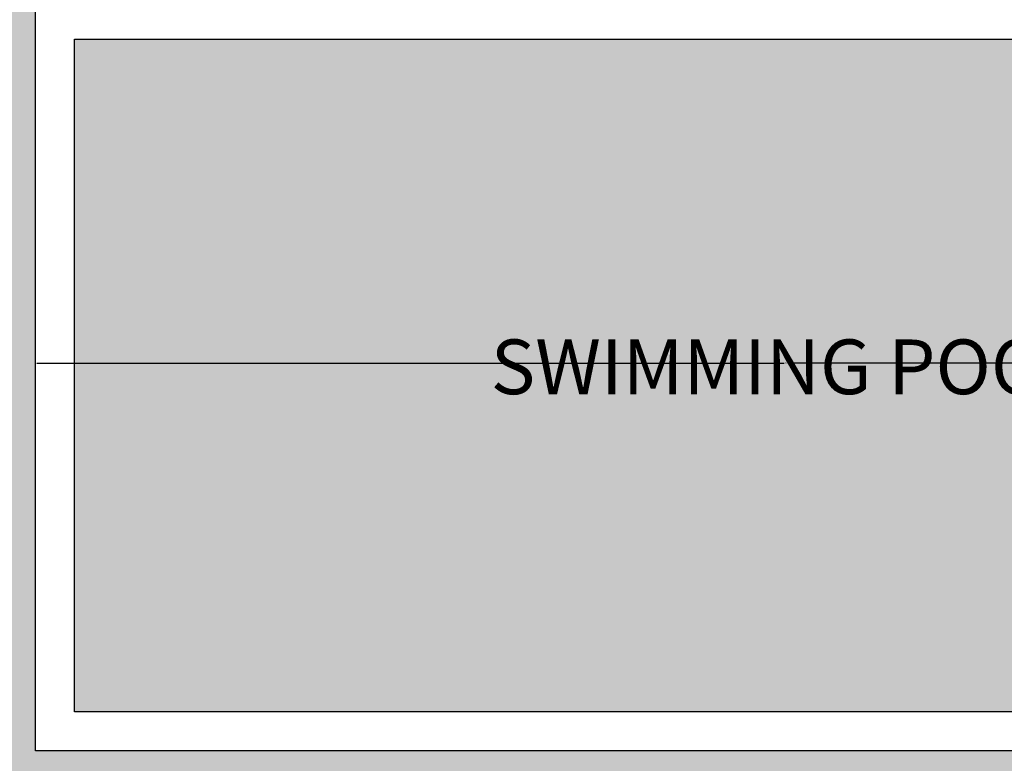
# Model space of a CAD drawing. Units: inches. Extents: x 84 to 1044, y -280 to 906.
# Tile 39 of 105: x 789 to 915, y -66 to 29. Entities that reach past the tile are written whole.
import ezdxf

# ---------------------------------------------------------------- set-up
doc = ezdxf.new("R2010")
doc.units = ezdxf.units.IN
for name, color, linetype, lineweight in [('A-ANNO-DIMS', 2, 'Continuous', 18), ('A-AREA-IDEN', 7, 'Continuous', 13), ('L-POOL', 151, 'Continuous', 25), ('L-POOL-PATT', 143, 'Continuous', 9)]:
    doc.layers.add(name, color=color, linetype=linetype, lineweight=lineweight)
doc.layers.add('L-PLNT-PATT', color=9, linetype='Continuous', lineweight=9, true_color=0xafd9aa)
doc.styles.add('1-100DIM', font='txt', dxfattribs={"height": 0.3})
doc.styles.get("Standard").update_dxf_attribs({"font": 'arial.ttf'})
doc.dimstyles.get("Standard").update_dxf_attribs({"dimtxt": 0.18, "dimasz": 0.18, "dimexe": 0.18, "dimexo": 0.0625, "dimgap": 0.09, "dimtad": 0, "dimtih": 1, "dimtoh": 1, "dimdec": 4, "dimzin": 0, "dimdsep": 46, "dimtxsty": 'Standard', "dimcen": 0.09, "dimadec": 0, "dimazin": 0, "dimtfac": 1, "dimtdec": 4, "dimtofl": 0, "dimtmove": 0, "dimatfit": 3, "dimfxl": 1, "dimtolj": 1, "dimtzin": 0, "dimarcsym": 0})

# ---------------------------------------------------------------- blocks, each defined once
blk = doc.blocks.new('*D67')
at = {"layer": 'A-ANNO-DIMS', "color": 0, "lineweight": -2, "transparency": 16777216}
for p, q in [((791.07, -64.82), (791.07, -15.1)), ((983.07, -64.82), (983.07, -15.1)), ((791.25, -15.28), (886.79, -15.28)), ((982.89, -15.28), (887.35, -15.28))]:
    blk.add_line(p, q, dxfattribs=at)
at = {"layer": 'A-ANNO-DIMS', "color": 0, "transparency": 16777216}
for points in [[(791.25, -15.25), (791.25, -15.31), (791.07, -15.28)], [(982.89, -15.25), (982.89, -15.31), (983.07, -15.28)]]:
    blk.add_solid(points, dxfattribs=at)
at = {"layer": 'Defpoints', "color": 0, "transparency": 16777216}
for p in [(983.07, -15.28), (791.07, -64.88), (983.07, -64.88)]:
    blk.add_point(p, dxfattribs=at)
at = {"layer": 'A-ANNO-DIMS', "color": 0, "transparency": 16777216, "insert": (887.07, -15.28), "char_height": 0.18, "attachment_point": 5}
blk.add_mtext('\\A1;192', dxfattribs=at)

msp = doc.modelspace()

# ---------------------------------------------------------------- hatches: boundary and pattern name
at = {"layer": 'L-PLNT-PATT', "transparency": 33554597}
h = msp.add_hatch(color=256, dxfattribs=at)
h.dxf.hatch_style = 1
h.paths.add_polyline_path([(791.074, 31.12), (791.074, 91.12), (743.074, 91.12), (674.074, 91.12), (674.074, 31.12), (650.074, 31.12), (650.074, -112.88), (983.074, -112.88), (983.074, -64.88), (791.074, -64.88)])
at = {"layer": 'L-POOL-PATT', "transparency": 33554567}
h = msp.add_hatch(color=256, dxfattribs=at)
h.dxf.hatch_style = 1
h.set_gradient(color1=(122, 175, 223), color2=(39, 118, 187), name='INVCYLINDER')
h.paths.add_polyline_path([(978.074, 26.12), (796.074, 26.12), (796.074, -59.88), (978.074, -59.88)])

# ---------------------------------------------------------------- linework, layer by layer
at = {"layer": 'L-POOL'}
for points in [[(791.074, 31.12), (983.074, 31.12), (983.074, -64.88), (791.074, -64.88)], [(796.074, 26.12), (978.074, 26.12), (978.074, -59.88), (796.074, -59.88)]]:
    msp.add_lwpolyline(points, close=True, dxfattribs=at)

# ---------------------------------------------------------------- texts
at = {"layer": 'A-AREA-IDEN', "insert": (844.983, -12.265), "char_height": 7, "attachment_point": 1, "style": '1-100DIM'}
msp.add_mtext_dynamic_manual_height_columns('{\\f@Malgun Gothic|b0|i0|c0|p34;  SWIMMING POOL}', width=95.90564, gutter_width=15.851, heights=[0], dxfattribs=at)

# ---------------------------------------------------------------- dimensions: what is measured, and where the dimension line sits
at = {"layer": 'A-ANNO-DIMS'}
dim = msp.add_linear_dim(base=(983.074, -15.28), p1=(791.074, -64.88), p2=(983.074, -64.88), angle=0, dimstyle='Standard', override={"dimdec": 0, "dimlfac": 1, "dimrnd": 0, "dimzin": 0, "dimdsep": 46, "dimlunit": 2}, dxfattribs=at)
dim.commit()
dim.dimension.update_dxf_attribs({"geometry": '*D67', "text_midpoint": (887.074, -15.28)})

doc.saveas('drawing.dxf')
